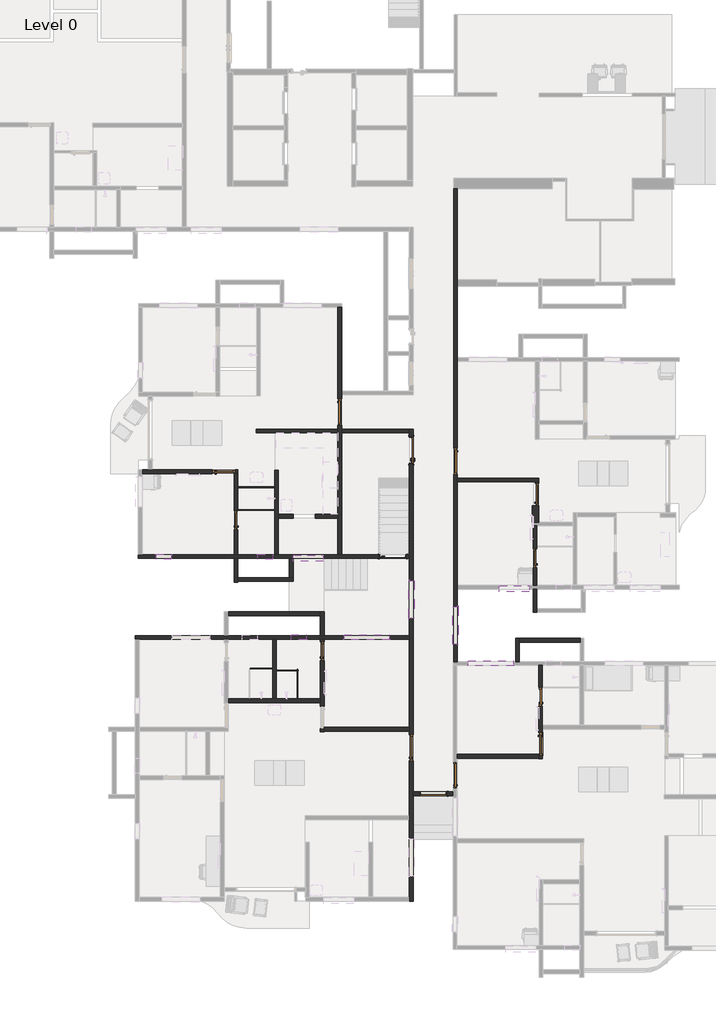
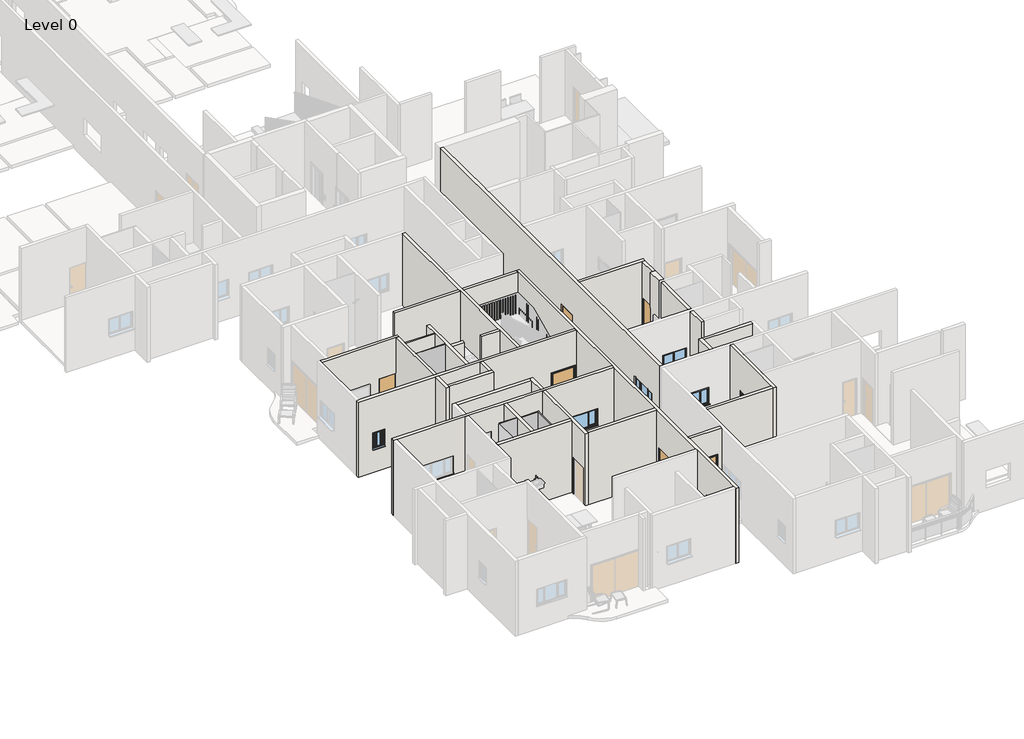
# One storey, part 2 of 14: 28 walls, 14 doors, 9 windows, 4 plates.
"""IFC4 building model written with IfcOpenShell, lengths in millimetres."""

from ifc_helpers import new_model, si_unit, frame, origin, origin_with_axes, place, context, project, spatial, polyline, outline, extrude, faceted_brep, transform, mapped, element, save
from components import doors_extsgl_flush_d1_30a970b5, doors_extsgl_flush_d1_11f69a25, doors_extsgl_flush_d2_fac1298c, doors_extsgl_flush_d2_5e0ff3e2, doors_extsgl_flush_d3_352cde1d, doors_extsgl_flush_d3_ba5ff989, doors_intsgl_3_75_1d728d0e, doors_intsgl_3_75_e7c258cb, system_panel_glazed_095a6893, system_panel_glazed_6806f88e, system_panel_glazed_1225bd09, system_panel_glazed_76c655e3, windows_concept_plain_dbl_4_d1e2e333, windows_sgl_plain_2_be143095, windows_tpl_variable_casement_2_47b04551, windows_tpl_variable_casement_5_ffad3fa3, windows_tpl_variable_casement_6_d811e495

model = new_model("IFC4")

# Units and contexts
model_context = context("Model", 3, world=origin())
ifc_project = project(units=[si_unit("LENGTHUNIT", "METRE", prefix="MILLI")], contexts=[model_context])

# Site, building, storey
site = spatial("IfcSite", under=ifc_project)
building = spatial("IfcBuilding", under=site)
storey = spatial("IfcBuildingStorey", under=building, Name="Level 0", Elevation=0.0)

# Doors
placement = place(None, origin())
doors_extsgl_flush_d1_shape = doors_extsgl_flush_d1_30a970b5(model_context)
element("IfcDoor", 1, ObjectType="Doors_ExtSgl_Flush : D1", at=placement, inside=storey, context=model_context, shape_type="MappedRepresentation", body=[
    mapped(doors_extsgl_flush_d1_shape, transform((-21668.1547508, 18097.2113431, 0.0), x_axis=(0.0, 1.0, 0.0), y_axis=(-1.0, 0.0, 0.0), z_axis=(0.0, 0.0, 1.0))),
])
element("IfcDoor", 2, ObjectType="Doors_ExtSgl_Flush : D1", at=placement, inside=storey, context=model_context, shape_type="MappedRepresentation", body=[
    mapped(doors_extsgl_flush_d1_shape, transform((-19869.6917798, 29735.6122683, 0.0), x_axis=(0.0, -1.0, 0.0), y_axis=(1.0, 0.0, 0.0), z_axis=(0.0, 0.0, 1.0))),
])
doors_extsgl_flush_d1_2_shape = doors_extsgl_flush_d1_11f69a25(model_context)
element("IfcDoor", 3, ObjectType="Doors_ExtSgl_Flush : D1", at=placement, inside=storey, context=model_context, shape_type="MappedRepresentation", body=[
    mapped(doors_extsgl_flush_d1_2_shape, transform((-19889.1949343, 16979.4762397, 0.0), x_axis=(0.0, 1.0, 0.0), y_axis=(-1.0, 0.0, 0.0), z_axis=(0.0, 0.0, 1.0))),
])
element("IfcDoor", 4, ObjectType="Doors_ExtSgl_Flush : D1", at=placement, inside=storey, context=model_context, shape_type="MappedRepresentation", body=[
    mapped(doors_extsgl_flush_d1_2_shape, transform((-24570.7800447, 31731.8982557, 0.0), x_axis=(0.0, -1.0, 0.0), y_axis=(1.0, 0.0, 0.0), z_axis=(0.0, 0.0, 1.0))),
])
doors_extsgl_flush_d2_shape = doors_extsgl_flush_d2_fac1298c(model_context)
element("IfcDoor", 5, ObjectType="Doors_ExtSgl_Flush : D2", at=placement, inside=storey, context=model_context, shape_type="MappedRepresentation", body=[
    mapped(doors_extsgl_flush_d2_shape, transform((-16561.3417798, 28376.6106683, 0.0), x_axis=(0.0, 1.0, 0.0), y_axis=(-1.0, 0.0, 0.0), z_axis=(0.0, 0.0, 1.0))),
])
doors_extsgl_flush_d2_2_shape = doors_extsgl_flush_d2_5e0ff3e2(model_context)
element("IfcDoor", 6, ObjectType="Doors_ExtSgl_Flush : D2", at=placement, inside=storey, context=model_context, shape_type="MappedRepresentation", body=[
    mapped(doors_extsgl_flush_d2_2_shape, transform((-16415.8741157, 18242.0106683, 0.0), x_axis=(0.0, -1.0, 0.0), y_axis=(1.0, 0.0, 0.0), z_axis=(0.0, 0.0, 1.0))),
])
element("IfcDoor", 7, ObjectType="Doors_ExtSgl_Flush : D2", at=placement, inside=storey, context=model_context, shape_type="MappedRepresentation", body=[
    mapped(doors_extsgl_flush_d2_2_shape, transform((-29288.9316447, 29306.9770746, 0.0), x_axis=(1.0, 0.0, 0.0), y_axis=(0.0, 1.0, 0.0), z_axis=(0.0, 0.0, 1.0))),
])
doors_extsgl_flush_d3_shape = doors_extsgl_flush_d3_352cde1d(model_context)
element("IfcDoor", 8, ObjectType="Doors_ExtSgl_Flush : D3", at=placement, inside=storey, context=model_context, shape_type="MappedRepresentation", body=[
    mapped(doors_extsgl_flush_d3_shape, transform((-25283.1553928, 22015.2629431, 0.0), x_axis=(0.0, 1.0, 0.0), y_axis=(-1.0, 0.0, 0.0), z_axis=(0.0, 0.0, 1.0))),
])
doors_extsgl_flush_d3_2_shape = doors_extsgl_flush_d3_ba5ff989(model_context)
element("IfcDoor", 9, ObjectType="Doors_ExtSgl_Flush : D3", at=placement, inside=storey, context=model_context, shape_type="MappedRepresentation", body=[
    mapped(doors_extsgl_flush_d3_2_shape, transform((-16415.8741157, 20166.1114683, 0.0), x_axis=(0.0, 1.0, 0.0), y_axis=(-1.0, 0.0, 0.0), z_axis=(0.0, 0.0, 1.0))),
])
element("IfcDoor", 10, ObjectType="Doors_ExtSgl_Flush : D3", at=placement, inside=storey, context=model_context, shape_type="MappedRepresentation", body=[
    mapped(doors_extsgl_flush_d3_2_shape, transform((-16639.8456172, 25796.359605, 0.0), x_axis=(0.0, 1.0, 0.0), y_axis=(-1.0, 0.0, 0.0), z_axis=(0.0, 0.0, 1.0))),
])
element("IfcDoor", 11, ObjectType="Doors_ExtSgl_Flush : D3", at=placement, inside=storey, context=model_context, shape_type="MappedRepresentation", body=[
    mapped(doors_extsgl_flush_d3_2_shape, transform((-28793.5300447, 27333.4986746, 0.0), x_axis=(0.0, 1.0, 0.0), y_axis=(-1.0, 0.0, 0.0), z_axis=(0.0, 0.0, 1.0))),
])
doors_intsgl_3_75_shape = doors_intsgl_3_75_1d728d0e(model_context)
element("IfcDoor", 12, ObjectType="Doors_IntSgl : 3.75'", at=placement, inside=storey, context=model_context, shape_type="MappedRepresentation", body=[
    mapped(doors_intsgl_3_75_shape, transform((-21668.1547508, 30185.5294818, 0.0), x_axis=(0.0, 1.0, 0.0), y_axis=(-1.0, 0.0, 0.0), z_axis=(0.0, 0.0, 1.0))),
])
element("IfcDoor", 13, ObjectType="Doors_IntSgl : 3.75'", at=placement, inside=storey, context=model_context, shape_type="MappedRepresentation", body=[
    mapped(doors_intsgl_3_75_shape, transform((-22417.4547508, 25858.9270746, 0.0), x_axis=(1.0, 0.0, 0.0), y_axis=(0.0, 1.0, 0.0), z_axis=(0.0, 0.0, 1.0))),
])
doors_intsgl_3_75_2_shape = doors_intsgl_3_75_e7c258cb(model_context)
element("IfcDoor", 14, ObjectType="Doors_IntSgl : 3.75'", at=placement, inside=storey, context=model_context, shape_type="MappedRepresentation", body=[
    mapped(doors_intsgl_3_75_2_shape, transform((-20778.6748425, 16225.043411, 508.0), x_axis=(-1.0, 0.0, 0.0), y_axis=(0.0, -1.0, 0.0), z_axis=(0.0, 0.0, 1.0))),
])

# Plates
system_panel_glazed_shape = system_panel_glazed_095a6893(model_context)
element("IfcPlate", 15, ObjectType="System Panel : Glazed", at=placement, inside=storey, context=model_context, shape_type="MappedRepresentation", body=[
    mapped(system_panel_glazed_shape, transform((-26257.0814081, 20677.4411882, 0.0), x_axis=(0.0, 1.0, 0.0), y_axis=(-1.0, 0.0, 0.0), z_axis=(0.0, 0.0, 1.0))),
])
system_panel_glazed_2_shape = system_panel_glazed_6806f88e(model_context)
element("IfcPlate", 16, ObjectType="System Panel : Glazed", at=placement, inside=storey, context=model_context, shape_type="MappedRepresentation", body=[
    mapped(system_panel_glazed_2_shape, transform((-27968.3995818, 27795.9116713, 0.0), x_axis=(-1.0, 0.0, 0.0), y_axis=(0.0, -1.0, 0.0), z_axis=(0.0, 0.0, 1.0))),
])
system_panel_glazed_3_shape = system_panel_glazed_1225bd09(model_context)
element("IfcPlate", 17, ObjectType="System Panel : Glazed", at=placement, inside=storey, context=model_context, shape_type="MappedRepresentation", body=[
    mapped(system_panel_glazed_3_shape, transform((-27760.3375826, 21274.3411882, 0.0), x_axis=(1.0, 0.0, 0.0), y_axis=(0.0, 1.0, 0.0), z_axis=(0.0, 0.0, 1.0))),
])
system_panel_glazed_4_shape = system_panel_glazed_76c655e3(model_context)
element("IfcPlate", 18, ObjectType="System Panel : Glazed", at=placement, inside=storey, context=model_context, shape_type="MappedRepresentation", body=[
    mapped(system_panel_glazed_4_shape, transform((-26705.9444157, 21274.3411882, 0.0), x_axis=(-1.0, 0.0, 0.0), y_axis=(0.0, -1.0, 0.0), z_axis=(0.0, 0.0, 1.0))),
])

# Walls
element("IfcWall", 19, ObjectType="W1", at=placement, inside=storey, context=model_context, shape_type="Brep", body=[
    faceted_brep([(-16492.0741157, 21442.5122683, 0.0), (-16492.0741157, 20547.1114683, 0.0), (-16492.0741157, 20547.1114683, 2110.0), (-16492.0741157, 19785.1114683, 2110.0), (-16492.0741157, 19785.1114683, 0.0), (-16492.0741157, 18699.2106683, 0.0), (-16492.0741157, 18699.2106683, 2110.0), (-16492.0741157, 17784.8106683, 2110.0), (-16492.0741157, 17784.8106683, 0.0), (-16492.0741157, 17670.5106683, 0.0), (-16492.0741157, 17651.5114683, 0.0), (-16492.0741157, 17651.5114683, 4000.0), (-16492.0741157, 17670.5106683, 4000.0), (-16492.0741157, 17822.9106683, 4000.0), (-16492.0741157, 21442.5122683, 4000.0), (-16339.6741157, 20547.1114683, 2110.0), (-16339.6741157, 20547.1114683, 0.0), (-16339.6741157, 21442.5122683, 0.0), (-16339.6741157, 21442.5122683, 4000.0), (-16339.6741157, 18997.7114683, 4000.0), (-16339.6741157, 18845.3114683, 4000.0), (-16339.6741157, 17651.5114683, 4000.0), (-16339.6741157, 17651.5114683, 0.0), (-16339.6741157, 17784.8106683, 0.0), (-16339.6741157, 17784.8106683, 2110.0), (-16339.6741157, 18699.2106683, 2110.0), (-16339.6741157, 18699.2106683, 0.0), (-16339.6741157, 18845.3114683, 0.0), (-16339.6741157, 18997.7114683, 0.0), (-16339.6741157, 19785.1114683, 0.0), (-16339.6741157, 19785.1114683, 2110.0)], [[[0, 1, 2, 3, 4, 5, 6, 7, 8, 9, 10, 11, 12, 13, 14]], [[15, 16, 17, 18, 19, 20, 21, 22, 23, 24, 25, 26, 27, 28, 29, 30]], [[10, 9, 8, 23, 22]], [[17, 16, 1, 0]], [[29, 28, 27, 26, 5, 4]], [[11, 10, 22, 21]], [[14, 13, 12, 11, 21, 20, 19, 18]], [[0, 14, 18, 17]], [[26, 25, 6, 5]], [[24, 23, 8, 7]], [[25, 24, 7, 6]], [[4, 3, 30, 29]], [[2, 1, 16, 15]], [[3, 2, 15, 30]]]),
])
element("IfcWall", 20, ObjectType="W1", at=placement, inside=storey, context=model_context, shape_type="Brep", body=[
    faceted_brep([(-19812.9949343, 17670.5106683, 0.0), (-16492.0741157, 17670.5106683, 0.0), (-16492.0741157, 17670.5106683, 4000.0), (-19812.9949343, 17670.5106683, 4000.0), (-19812.9949343, 17822.9106683, 0.0), (-19812.9949343, 17822.9106683, 4000.0), (-16492.0741157, 17822.9106683, 4000.0), (-16492.0741157, 17822.9106683, 0.0), (-16492.0741157, 17784.8106683, 0.0)], [[[0, 1, 2, 3]], [[4, 5, 6, 7]], [[1, 0, 4, 7, 8]], [[3, 2, 6, 5]], [[0, 3, 5, 4]], [[2, 1, 8, 7, 6]]]),
])
element("IfcWall", 21, ObjectType="W1", at=placement, inside=storey, context=model_context, shape_type="SweptSolid", body=[
    extrude(outline(polyline([(0.0, -21591.9547508), (0.0, -19965.3949343), (4000.0, -19965.3949343), (4000.0, -21591.9547508), (0.0, -21591.9547508)]), holes=[polyline([(508.0, -21350.1748425), (2641.6, -21350.1748425), (2641.6, -20207.1748425), (508.0, -20207.1748425), (508.0, -21350.1748425)])]), frame((0.0, 16148.843411, 0.0), z_axis=(0.0, 1.0, 0.0), x_axis=(0.0, 0.0, 1.0)), (0.0, 0.0, 1.0), 152.4),
])
element("IfcWall", 22, ObjectType="W1", at=placement, inside=storey, context=model_context, shape_type="Brep", body=[
    faceted_brep([(-21591.9547508, 31036.4294818, 4000.0), (-21591.9547508, 16301.243411, 4000.0), (-21591.9547508, 16148.843411, 4000.0), (-21591.9547508, 11859.4294818, 4000.0), (-21591.9547508, 11859.4294818, 0.0), (-21591.9547508, 16148.843411, 0.0), (-21591.9547508, 16301.243411, 0.0), (-21591.9547508, 17563.8113431, 0.0), (-21591.9547508, 17563.8113431, 2110.0), (-21591.9547508, 18630.6113431, 2110.0), (-21591.9547508, 18630.6113431, 0.0), (-21591.9547508, 29614.0294818, 0.0), (-21591.9547508, 29614.0294818, 2133.6), (-21591.9547508, 30757.0294818, 2133.6), (-21591.9547508, 30757.0294818, 0.0), (-21591.9547508, 31036.4294818, 0.0), (-21591.9547508, 14397.2288681, 2110.0), (-21591.9547508, 14397.2288681, 1200.0), (-21591.9547508, 12873.2288681, 1200.0), (-21591.9547508, 12873.2288681, 2110.0), (-21591.9547508, 24887.7601529, 2110.0), (-21591.9547508, 24887.7601529, 1200.0), (-21591.9547508, 23363.7601529, 1200.0), (-21591.9547508, 23363.7601529, 2110.0), (-21744.3547508, 11859.4294818, 4000.0), (-21744.3547508, 12011.8294818, 4000.0), (-21744.3547508, 15172.0304681, 4000.0), (-21744.3547508, 15324.4304681, 4000.0), (-21744.3547508, 18770.4129431, 4000.0), (-21744.3547508, 18922.8129431, 4000.0), (-21744.3547508, 22500.1601529, 4000.0), (-21744.3547508, 22652.5601529, 4000.0), (-21744.3547508, 25782.7270746, 4000.0), (-21744.3547508, 25935.1270746, 4000.0), (-21744.3547508, 30884.0294818, 4000.0), (-21744.3547508, 31036.4294818, 4000.0), (-21744.3547508, 31036.4294818, 0.0), (-21744.3547508, 30884.0294818, 0.0), (-21744.3547508, 30757.0294818, 0.0), (-21744.3547508, 30757.0294818, 2133.6), (-21744.3547508, 29614.0294818, 2133.6), (-21744.3547508, 29614.0294818, 0.0), (-21744.3547508, 25935.1270746, 0.0), (-21744.3547508, 25782.7270746, 0.0), (-21744.3547508, 22652.5601529, 0.0), (-21744.3547508, 22500.1601529, 0.0), (-21744.3547508, 18922.8129431, 0.0), (-21744.3547508, 18770.4129431, 0.0), (-21744.3547508, 18630.6113431, 0.0), (-21744.3547508, 18630.6113431, 2110.0), (-21744.3547508, 17563.8113431, 2110.0), (-21744.3547508, 17563.8113431, 0.0), (-21744.3547508, 15324.4304681, 0.0), (-21744.3547508, 15172.0304681, 0.0), (-21744.3547508, 12011.8294818, 0.0), (-21744.3547508, 11859.4294818, 0.0), (-21744.3547508, 14397.2288681, 2110.0), (-21744.3547508, 12873.2288681, 2110.0), (-21744.3547508, 12873.2288681, 1200.0), (-21744.3547508, 14397.2288681, 1200.0), (-21744.3547508, 24887.7601529, 2110.0), (-21744.3547508, 23363.7601529, 2110.0), (-21744.3547508, 23363.7601529, 1200.0), (-21744.3547508, 24887.7601529, 1200.0)], [[[0, 1, 2, 3, 4, 5, 6, 7, 8, 9, 10, 11, 12, 13, 14, 15], [16, 17, 18, 19], [20, 21, 22, 23]], [[24, 25, 26, 27, 28, 29, 30, 31, 32, 33, 34, 35, 36, 37, 38, 39, 40, 41, 42, 43, 44, 45, 46, 47, 48, 49, 50, 51, 52, 53, 54, 55], [56, 57, 58, 59], [60, 61, 62, 63]], [[4, 55, 54, 53, 52, 51, 7, 6, 5]], [[36, 15, 14, 38, 37]], [[10, 48, 47, 46, 45, 44, 43, 42, 41, 11]], [[3, 2, 1, 0, 35, 34, 33, 32, 31, 30, 29, 28, 27, 26, 25, 24]], [[4, 3, 24, 55]], [[0, 15, 36, 35]], [[51, 50, 8, 7]], [[49, 48, 10, 9]], [[50, 49, 9, 8]], [[17, 16, 56, 59]], [[18, 17, 59, 58]], [[19, 18, 58, 57]], [[16, 19, 57, 56]], [[13, 39, 38, 14]], [[39, 13, 12, 40]], [[40, 12, 11, 41]], [[21, 20, 60, 63]], [[22, 21, 63, 62]], [[23, 22, 62, 61]], [[20, 23, 61, 60]]]),
])
element("IfcWall", 23, ObjectType="W1", at=placement, inside=storey, context=model_context, shape_type="Brep", body=[
    faceted_brep([(-21744.3547508, 22652.5601529, 0.0), (-25206.9553928, 22652.5601529, 0.0), (-25359.3553928, 22652.5601529, 0.0), (-29107.0280604, 22652.5601529, 0.0), (-29259.4280604, 22652.5601529, 0.0), (-32875.9555508, 22652.5601529, 0.0), (-32875.9555508, 22652.5601529, 4000.0), (-29259.4280604, 22652.5601529, 4000.0), (-29107.0280604, 22652.5601529, 4000.0), (-25359.3553928, 22652.5601529, 4000.0), (-25206.9553928, 22652.5601529, 4000.0), (-21744.3547508, 22652.5601529, 4000.0), (-28539.2090234, 22652.5601529, 2738.9328), (-28539.2090234, 22652.5601529, 1828.9328), (-27929.6090234, 22652.5601529, 1828.9328), (-27929.6090234, 22652.5601529, 2738.9328), (-26545.2074234, 22652.5601529, 2738.9328), (-26545.2074234, 22652.5601529, 1828.9328), (-25935.6074234, 22652.5601529, 1828.9328), (-25935.6074234, 22652.5601529, 2738.9328), (-31387.0322871, 22652.5601529, 2110.0), (-31387.0322871, 22652.5601529, 1200.0), (-29863.0322871, 22652.5601529, 1200.0), (-29863.0322871, 22652.5601529, 2110.0), (-24398.7563508, 22652.5601529, 2110.0), (-24398.7563508, 22652.5601529, 1200.0), (-22569.9563508, 22652.5601529, 1200.0), (-22569.9563508, 22652.5601529, 2110.0), (-21744.3547508, 22500.1601529, 0.0), (-21744.3547508, 22500.1601529, 4000.0), (-25206.9553928, 22500.1601529, 4000.0), (-25359.3553928, 22500.1601529, 4000.0), (-27154.8074234, 22500.1601529, 4000.0), (-27307.2074234, 22500.1601529, 4000.0), (-29107.0280604, 22500.1601529, 4000.0), (-29259.4280604, 22500.1601529, 4000.0), (-32723.5555508, 22500.1601529, 4000.0), (-32875.9555508, 22500.1601529, 4000.0), (-32875.9555508, 22500.1601529, 0.0), (-32723.5555508, 22500.1601529, 0.0), (-29259.4280604, 22500.1601529, 0.0), (-29107.0280604, 22500.1601529, 0.0), (-27307.2074234, 22500.1601529, 0.0), (-27154.8074234, 22500.1601529, 0.0), (-25359.3553928, 22500.1601529, 0.0), (-25206.9553928, 22500.1601529, 0.0), (-28539.2090234, 22500.1601529, 2738.9328), (-27929.6090234, 22500.1601529, 2738.9328), (-27929.6090234, 22500.1601529, 1828.9328), (-28539.2090234, 22500.1601529, 1828.9328), (-26545.2074234, 22500.1601529, 2738.9328), (-25935.6074234, 22500.1601529, 2738.9328), (-25935.6074234, 22500.1601529, 1828.9328), (-26545.2074234, 22500.1601529, 1828.9328), (-31387.0322871, 22500.1601529, 2110.0), (-29863.0322871, 22500.1601529, 2110.0), (-29863.0322871, 22500.1601529, 1200.0), (-31387.0322871, 22500.1601529, 1200.0), (-24398.7563508, 22500.1601529, 2110.0), (-22569.9563508, 22500.1601529, 2110.0), (-22569.9563508, 22500.1601529, 1200.0), (-24398.7563508, 22500.1601529, 1200.0)], [[[0, 1, 2, 3, 4, 5, 6, 7, 8, 9, 10, 11], [12, 13, 14, 15], [16, 17, 18, 19], [20, 21, 22, 23], [24, 25, 26, 27]], [[28, 29, 30, 31, 32, 33, 34, 35, 36, 37, 38, 39, 40, 41, 42, 43, 44, 45], [46, 47, 48, 49], [50, 51, 52, 53], [54, 55, 56, 57], [58, 59, 60, 61]], [[5, 4, 3, 2, 1, 0, 28, 45, 44, 43, 42, 41, 40, 39, 38]], [[11, 10, 9, 8, 7, 6, 37, 36, 35, 34, 33, 32, 31, 30, 29]], [[0, 11, 29, 28]], [[6, 5, 38, 37]], [[13, 12, 46, 49]], [[14, 13, 49, 48]], [[15, 14, 48, 47]], [[12, 15, 47, 46]], [[17, 16, 50, 53]], [[18, 17, 53, 52]], [[19, 18, 52, 51]], [[16, 19, 51, 50]], [[21, 20, 54, 57]], [[22, 21, 57, 56]], [[23, 22, 56, 55]], [[20, 23, 55, 54]], [[25, 24, 58, 61]], [[26, 25, 61, 60]], [[27, 26, 60, 59]], [[24, 27, 59, 58]]]),
])
element("IfcWall", 24, ObjectType="W1", at=placement, inside=storey, context=model_context, shape_type="Brep", body=[
    faceted_brep([(-29107.0280604, 19928.1411882, 0.0), (-25359.3553928, 19928.1411882, 0.0), (-25359.3553928, 19928.1411882, 4000.0), (-29107.0280604, 19928.1411882, 4000.0), (-29107.0280604, 20080.5411882, 0.0), (-29107.0280604, 20080.5411882, 4000.0), (-27307.2074234, 20080.5411882, 4000.0), (-27154.8074234, 20080.5411882, 4000.0), (-25359.3553928, 20080.5411882, 4000.0), (-25359.3553928, 20080.5411882, 0.0), (-27154.8074234, 20080.5411882, 0.0), (-27307.2074234, 20080.5411882, 0.0)], [[[0, 1, 2, 3]], [[4, 5, 6, 7, 8, 9, 10, 11]], [[1, 0, 4, 11, 10, 9]], [[3, 2, 8, 7, 6, 5]], [[0, 3, 5, 4]], [[2, 1, 9, 8]]]),
])
element("IfcWall", 25, ObjectType="W1", at=placement, inside=storey, context=model_context, shape_type="SweptSolid", body=[
    extrude(outline(polyline([(-27307.2074234, 20080.5411882), (-27307.2074234, 22500.1601529), (-27154.8074234, 22500.1601529), (-27154.8074234, 20080.5411882), (-27307.2074234, 20080.5411882)])), origin_with_axes(), (0.0, 0.0, 1.0), 4000.0),
])
element("IfcWall", 26, ObjectType="W1", at=placement, inside=storey, context=model_context, shape_type="Brep", body=[
    faceted_brep([(-25359.3553928, 18745.0129431, 0.0), (-25359.3553928, 18745.0129431, 4000.0), (-25359.3553928, 19928.1411882, 4000.0), (-25359.3553928, 20080.5411882, 4000.0), (-25359.3553928, 22500.1601529, 4000.0), (-25359.3553928, 22500.1601529, 0.0), (-25359.3553928, 22396.2629431, 0.0), (-25359.3553928, 22396.2629431, 2110.0), (-25359.3553928, 21634.2629431, 2110.0), (-25359.3553928, 21634.2629431, 0.0), (-25359.3553928, 20080.5411882, 0.0), (-25359.3553928, 19928.1411882, 0.0), (-25359.3553928, 19787.3762656, 0.0), (-25359.3553928, 19787.3762656, 2110.0), (-25359.3553928, 18872.9762656, 2110.0), (-25359.3553928, 18872.9762656, 0.0), (-25206.9553928, 18745.0129431, 4000.0), (-25206.9553928, 18745.0129431, 0.0), (-25206.9553928, 18770.4129431, 0.0), (-25206.9553928, 18872.9762656, 0.0), (-25206.9553928, 18872.9762656, 2110.0), (-25206.9553928, 19787.3762656, 2110.0), (-25206.9553928, 19787.3762656, 0.0), (-25206.9553928, 21634.2629431, 0.0), (-25206.9553928, 21634.2629431, 2110.0), (-25206.9553928, 22396.2629431, 2110.0), (-25206.9553928, 22396.2629431, 0.0), (-25206.9553928, 22500.1601529, 0.0), (-25206.9553928, 22500.1601529, 4000.0), (-25206.9553928, 18922.8129431, 4000.0), (-25206.9553928, 18770.4129431, 4000.0)], [[[0, 1, 2, 3, 4, 5, 6, 7, 8, 9, 10, 11, 12, 13, 14, 15]], [[16, 17, 18, 19, 20, 21, 22, 23, 24, 25, 26, 27, 28, 29, 30]], [[17, 0, 15, 19, 18]], [[22, 12, 11, 10, 9, 23]], [[26, 6, 5, 27]], [[1, 0, 17, 16]], [[1, 16, 30, 29, 28, 4, 3, 2]], [[5, 4, 28, 27]], [[22, 21, 13, 12]], [[20, 19, 15, 14]], [[21, 20, 14, 13]], [[9, 8, 24, 23]], [[7, 6, 26, 25]], [[8, 7, 25, 24]]]),
    faceted_brep([(-25359.3553928, 23611.1411882, 4000.0), (-25359.3553928, 23611.1411882, 0.0), (-25359.3553928, 23458.7411882, 0.0), (-25359.3553928, 22652.5601529, 0.0), (-25359.3553928, 22652.5601529, 4000.0), (-25359.3553928, 23458.7411882, 4000.0), (-25206.9553928, 23611.1411882, 0.0), (-25206.9553928, 23611.1411882, 4000.0), (-25206.9553928, 22652.5601529, 4000.0), (-25206.9553928, 22652.5601529, 0.0)], [[[0, 1, 2, 3, 4, 5]], [[6, 7, 8, 9]], [[1, 6, 9, 3, 2]], [[7, 0, 5, 4, 8]], [[4, 3, 9, 8]], [[1, 0, 7, 6]]]),
])
element("IfcWall", 27, ObjectType="W1", at=placement, inside=storey, context=model_context, shape_type="Brep", body=[
    faceted_brep([(-25206.9553928, 18770.4129431, 0.0), (-21744.3547508, 18770.4129431, 0.0), (-21744.3547508, 18770.4129431, 4000.0), (-25206.9553928, 18770.4129431, 4000.0), (-25206.9553928, 18922.8129431, 0.0), (-25206.9553928, 18922.8129431, 4000.0), (-21744.3547508, 18922.8129431, 4000.0), (-21744.3547508, 18922.8129431, 0.0), (-25206.9553928, 18872.9762656, 0.0)], [[[0, 1, 2, 3]], [[4, 5, 6, 7]], [[1, 0, 8, 4, 7]], [[3, 2, 6, 5]], [[2, 1, 7, 6]], [[0, 3, 5, 4, 8]]]),
])
element("IfcWall", 28, ObjectType="W1", at=placement, inside=storey, context=model_context, shape_type="Brep", body=[
    faceted_brep([(-32762.2800447, 25935.1270746, 4000.0), (-32609.8800447, 25935.1270746, 4000.0), (-28869.7300447, 25935.1270746, 4000.0), (-28717.3300447, 25935.1270746, 4000.0), (-27219.4691188, 25935.1270746, 4000.0), (-27067.0691188, 25935.1270746, 4000.0), (-24646.9800447, 25935.1270746, 4000.0), (-24494.5800447, 25935.1270746, 4000.0), (-21744.3547508, 25935.1270746, 4000.0), (-21744.3547508, 25935.1270746, 0.0), (-21845.9547508, 25935.1270746, 0.0), (-21845.9547508, 25935.1270746, 2133.6), (-22988.9547508, 25935.1270746, 2133.6), (-22988.9547508, 25935.1270746, 0.0), (-24494.5800447, 25935.1270746, 0.0), (-24646.9800447, 25935.1270746, 0.0), (-27067.0691188, 25935.1270746, 0.0), (-27219.4691188, 25935.1270746, 0.0), (-28717.3300447, 25935.1270746, 0.0), (-28869.7300447, 25935.1270746, 0.0), (-32609.8800447, 25935.1270746, 0.0), (-32762.2800447, 25935.1270746, 0.0), (-31416.0800447, 25935.1270746, 2110.0), (-32025.6800447, 25935.1270746, 2110.0), (-32025.6800447, 25935.1270746, 1200.0), (-31416.0800447, 25935.1270746, 1200.0), (-25247.4245818, 25935.1270746, 2110.0), (-26466.6245818, 25935.1270746, 2110.0), (-26466.6245818, 25935.1270746, 1200.0), (-25247.4245818, 25935.1270746, 1200.0), (-27295.6691188, 25935.1270746, 1828.9328), (-27295.6691188, 25935.1270746, 2738.9328), (-27905.2691188, 25935.1270746, 2738.9328), (-27905.2691188, 25935.1270746, 1828.9328), (-21744.3547508, 25782.7270746, 4000.0), (-26469.4300447, 25782.7270746, 4000.0), (-26621.8300447, 25782.7270746, 4000.0), (-28717.3300447, 25782.7270746, 4000.0), (-28869.7300447, 25782.7270746, 4000.0), (-32762.2800447, 25782.7270746, 4000.0), (-32762.2800447, 25782.7270746, 0.0), (-28869.7300447, 25782.7270746, 0.0), (-28717.3300447, 25782.7270746, 0.0), (-26621.8300447, 25782.7270746, 0.0), (-26469.4300447, 25782.7270746, 0.0), (-22988.9547508, 25782.7270746, 0.0), (-22988.9547508, 25782.7270746, 2133.6), (-21845.9547508, 25782.7270746, 2133.6), (-21845.9547508, 25782.7270746, 0.0), (-21744.3547508, 25782.7270746, 0.0), (-31416.0800447, 25782.7270746, 2110.0), (-31416.0800447, 25782.7270746, 1200.0), (-32025.6800447, 25782.7270746, 1200.0), (-32025.6800447, 25782.7270746, 2110.0), (-25247.4245818, 25782.7270746, 2110.0), (-25247.4245818, 25782.7270746, 1200.0), (-26466.6245818, 25782.7270746, 1200.0), (-26466.6245818, 25782.7270746, 2110.0), (-27295.6691188, 25782.7270746, 2738.9328), (-27295.6691188, 25782.7270746, 1828.9328), (-27905.2691188, 25782.7270746, 1828.9328), (-27905.2691188, 25782.7270746, 2738.9328)], [[[0, 1, 2, 3, 4, 5, 6, 7, 8, 9, 10, 11, 12, 13, 14, 15, 16, 17, 18, 19, 20, 21], [22, 23, 24, 25], [26, 27, 28, 29], [30, 31, 32, 33]], [[34, 35, 36, 37, 38, 39, 40, 41, 42, 43, 44, 45, 46, 47, 48, 49], [50, 51, 52, 53], [54, 55, 56, 57], [58, 59, 60, 61]], [[40, 21, 20, 19, 18, 17, 16, 15, 14, 13, 45, 44, 43, 42, 41]], [[9, 49, 48, 10]], [[8, 7, 6, 5, 4, 3, 2, 1, 0, 39, 38, 37, 36, 35, 34]], [[0, 21, 40, 39]], [[51, 50, 22, 25]], [[52, 51, 25, 24]], [[53, 52, 24, 23]], [[50, 53, 23, 22]], [[55, 54, 26, 29]], [[56, 55, 29, 28]], [[57, 56, 28, 27]], [[54, 57, 27, 26]], [[59, 58, 31, 30]], [[60, 59, 30, 33]], [[61, 60, 33, 32]], [[58, 61, 32, 31]], [[9, 8, 34, 49]], [[47, 11, 10, 48]], [[11, 47, 46, 12]], [[12, 46, 45, 13]]]),
])
element("IfcWall", 29, ObjectType="W1", at=placement, inside=storey, context=model_context, shape_type="Brep", body=[
    faceted_brep([(-24494.5800447, 25935.1270746, 0.0), (-24494.5800447, 30884.0294818, 0.0), (-24494.5800447, 31036.4294818, 0.0), (-24494.5800447, 31198.4982557, 0.0), (-24494.5800447, 31198.4982557, 2110.0), (-24494.5800447, 32265.2982557, 2110.0), (-24494.5800447, 32265.2982557, 0.0), (-24494.5800447, 32430.4998557, 0.0), (-24494.5800447, 32582.8998557, 0.0), (-24494.5800447, 35984.9800488, 0.0), (-24494.5800447, 35984.9800488, 4000.0), (-24494.5800447, 32582.8998557, 4000.0), (-24494.5800447, 32430.4998557, 4000.0), (-24494.5800447, 31036.4294818, 4000.0), (-24494.5800447, 30884.0294818, 4000.0), (-24494.5800447, 25935.1270746, 4000.0), (-24646.9800447, 31198.4982557, 2110.0), (-24646.9800447, 31198.4982557, 0.0), (-24646.9800447, 31036.4294818, 0.0), (-24646.9800447, 30884.0294818, 0.0), (-24646.9800447, 27580.0116713, 0.0), (-24646.9800447, 27427.6116713, 0.0), (-24646.9800447, 25935.1270746, 0.0), (-24646.9800447, 25935.1270746, 4000.0), (-24646.9800447, 27427.6116713, 4000.0), (-24646.9800447, 27580.0116713, 4000.0), (-24646.9800447, 30884.0294818, 4000.0), (-24646.9800447, 31036.4294818, 4000.0), (-24646.9800447, 35984.9800488, 4000.0), (-24646.9800447, 35984.9800488, 0.0), (-24646.9800447, 32265.2982557, 0.0), (-24646.9800447, 32265.2982557, 2110.0)], [[[0, 1, 2, 3, 4, 5, 6, 7, 8, 9, 10, 11, 12, 13, 14, 15]], [[16, 17, 18, 19, 20, 21, 22, 23, 24, 25, 26, 27, 28, 29, 30, 31]], [[30, 29, 9, 8, 7, 6]], [[22, 21, 20, 19, 18, 17, 3, 2, 1, 0]], [[15, 14, 13, 12, 11, 10, 28, 27, 26, 25, 24, 23]], [[0, 15, 23, 22]], [[10, 9, 29, 28]], [[6, 5, 31, 30]], [[4, 3, 17, 16]], [[5, 4, 16, 31]]]),
])
element("IfcWall", 30, ObjectType="W1", at=placement, inside=storey, context=model_context, shape_type="SweptSolid", body=[
    extrude(outline(polyline([(-27961.1063508, 30884.0294818), (-27961.1063508, 31036.4294818), (-24646.9800447, 31036.4294818), (-24646.9800447, 30884.0294818), (-27961.1063508, 30884.0294818)])), origin_with_axes(), (0.0, 0.0, 1.0), 4000.0),
    extrude(outline(polyline([(-21744.3547508, 31036.4294818), (-21744.3547508, 30884.0294818), (-24494.5800447, 30884.0294818), (-24494.5800447, 31036.4294818), (-21744.3547508, 31036.4294818)])), origin_with_axes(), (0.0, 0.0, 1.0), 4000.0),
])
element("IfcWall", 31, ObjectType="W1", at=placement, inside=storey, context=model_context, shape_type="Brep", body=[
    faceted_brep([(-28831.7316447, 29230.7770746, 2110.0), (-28831.7316447, 29230.7770746, 0.0), (-28717.3300447, 29230.7770746, 0.0), (-28717.3300447, 29230.7770746, 4000.0), (-28869.7300447, 29230.7770746, 4000.0), (-32609.8800447, 29230.7770746, 4000.0), (-32609.8800447, 29230.7770746, 0.0), (-29746.1316447, 29230.7770746, 0.0), (-29746.1316447, 29230.7770746, 2110.0), (-28717.3300447, 29383.1770746, 0.0), (-28831.7316447, 29383.1770746, 0.0), (-28831.7316447, 29383.1770746, 2110.0), (-29746.1316447, 29383.1770746, 2110.0), (-29746.1316447, 29383.1770746, 0.0), (-32203.4800447, 29383.1770746, 0.0), (-32355.8800447, 29383.1770746, 0.0), (-32609.8800447, 29383.1770746, 0.0), (-32609.8800447, 29383.1770746, 4000.0), (-32355.8800447, 29383.1770746, 4000.0), (-32203.4800447, 29383.1770746, 4000.0), (-28717.3300447, 29383.1770746, 4000.0)], [[[0, 1, 2, 3, 4, 5, 6, 7, 8]], [[9, 10, 11, 12, 13, 14, 15, 16, 17, 18, 19, 20]], [[7, 6, 16, 15, 14, 13]], [[2, 1, 10, 9]], [[5, 4, 3, 20, 19, 18, 17]], [[6, 5, 17, 16]], [[3, 2, 9, 20]], [[13, 12, 8, 7]], [[11, 10, 1, 0]], [[12, 11, 0, 8]]]),
])
element("IfcWall", 32, ObjectType="W1", at=placement, inside=storey, context=model_context, shape_type="Brep", body=[
    faceted_brep([(-28869.7300447, 24823.8262746, 0.0), (-28869.7300447, 24823.8262746, 4000.0), (-28869.7300447, 25782.7270746, 4000.0), (-28869.7300447, 25782.7270746, 0.0), (-28717.3300447, 24823.8262746, 4000.0), (-28717.3300447, 24823.8262746, 0.0), (-28717.3300447, 24849.2262746, 0.0), (-28717.3300447, 25001.6262746, 0.0), (-28717.3300447, 25782.7270746, 0.0), (-28717.3300447, 25782.7270746, 4000.0), (-28717.3300447, 25001.6262746, 4000.0), (-28717.3300447, 24849.2262746, 4000.0)], [[[0, 1, 2, 3]], [[4, 5, 6, 7, 8, 9, 10, 11]], [[5, 0, 3, 8, 7, 6]], [[1, 0, 5, 4]], [[1, 4, 11, 10, 9, 2]], [[3, 2, 9, 8]]]),
    faceted_brep([(-28869.7300447, 29230.7770746, 4000.0), (-28869.7300447, 29230.7770746, 0.0), (-28869.7300447, 27714.4986746, 0.0), (-28869.7300447, 27714.4986746, 2110.0), (-28869.7300447, 26952.4986746, 2110.0), (-28869.7300447, 26952.4986746, 0.0), (-28869.7300447, 25935.1270746, 0.0), (-28869.7300447, 25935.1270746, 4000.0), (-28717.3300447, 29230.7770746, 0.0), (-28717.3300447, 29230.7770746, 4000.0), (-28717.3300447, 28703.6762746, 4000.0), (-28717.3300447, 28654.2986746, 4000.0), (-28717.3300447, 25935.1270746, 4000.0), (-28717.3300447, 25935.1270746, 0.0), (-28717.3300447, 26952.4986746, 0.0), (-28717.3300447, 26952.4986746, 2110.0), (-28717.3300447, 27714.4986746, 2110.0), (-28717.3300447, 27714.4986746, 0.0), (-28717.3300447, 28654.2986746, 0.0), (-28717.3300447, 28703.6762746, 0.0), (-28831.7316447, 29230.7770746, 0.0)], [[[0, 1, 2, 3, 4, 5, 6, 7]], [[8, 9, 10, 11, 12, 13, 14, 15, 16, 17, 18, 19]], [[1, 20, 8, 19, 18, 17, 2]], [[5, 14, 13, 6]], [[9, 0, 7, 12, 11, 10]], [[1, 0, 9, 8, 20]], [[7, 6, 13, 12]], [[5, 4, 15, 14]], [[3, 2, 17, 16]], [[4, 3, 16, 15]]]),
])
element("IfcWall", 33, ObjectType="W1", at=placement, inside=storey, context=model_context, shape_type="Brep", body=[
    faceted_brep([(-28717.3300447, 24849.2262746, 0.0), (-26469.4300447, 24849.2262746, 0.0), (-26469.4300447, 24849.2262746, 4000.0), (-28717.3300447, 24849.2262746, 4000.0), (-28717.3300447, 25001.6262746, 0.0), (-28717.3300447, 25001.6262746, 4000.0), (-26621.8300447, 25001.6262746, 4000.0), (-26469.4300447, 25001.6262746, 4000.0), (-26469.4300447, 25001.6262746, 0.0), (-26621.8300447, 25001.6262746, 0.0)], [[[0, 1, 2, 3]], [[4, 5, 6, 7, 8, 9]], [[1, 0, 4, 9, 8]], [[3, 2, 7, 6, 5]], [[0, 3, 5, 4]], [[2, 1, 8, 7]]]),
])
element("IfcWall", 34, ObjectType="W1", at=placement, inside=storey, context=model_context, shape_type="SweptSolid", body=[
    extrude(outline(polyline([(-26469.4300447, 25782.7270746), (-26469.4300447, 25001.6262746), (-26621.8300447, 25001.6262746), (-26621.8300447, 25782.7270746), (-26469.4300447, 25782.7270746)])), origin_with_axes(), (0.0, 0.0, 1.0), 4000.0),
])
element("IfcWall", 35, ObjectType="W1", at=placement, inside=storey, context=model_context, shape_type="Brep", body=[
    faceted_brep([(-27219.4691188, 29369.8991476, 0.0), (-27219.4691188, 28703.6762746, 0.0), (-27219.4691188, 28654.2986746, 0.0), (-27219.4691188, 25935.1270746, 0.0), (-27219.4691188, 25935.1270746, 4000.0), (-27219.4691188, 28654.2986746, 4000.0), (-27219.4691188, 28703.6762746, 4000.0), (-27219.4691188, 29369.8991476, 4000.0), (-27067.0691188, 29369.8991476, 0.0), (-27067.0691188, 29369.8991476, 4000.0), (-27067.0691188, 27580.0116713, 4000.0), (-27067.0691188, 27427.6116713, 4000.0), (-27067.0691188, 25935.1270746, 4000.0), (-27067.0691188, 25935.1270746, 0.0), (-27067.0691188, 27427.6116713, 0.0), (-27067.0691188, 27580.0116713, 0.0)], [[[0, 1, 2, 3, 4, 5, 6, 7]], [[8, 9, 10, 11, 12, 13, 14, 15]], [[3, 2, 1, 0, 8, 15, 14, 13]], [[7, 6, 5, 4, 12, 11, 10, 9]], [[0, 7, 9, 8]], [[4, 3, 13, 12]]]),
])
element("IfcWall", 36, ObjectType="W1", at=placement, inside=storey, context=model_context, shape_type="Brep", body=[
    faceted_brep([(-19793.4917798, 21594.9122683, 0.0), (-19793.4917798, 24541.3122683, 0.0), (-19793.4917798, 24693.7122683, 0.0), (-19793.4917798, 28897.4122683, 0.0), (-19793.4917798, 29049.8122683, 0.0), (-19793.4917798, 29202.2122683, 0.0), (-19793.4917798, 29202.2122683, 2110.0), (-19793.4917798, 30269.0122683, 2110.0), (-19793.4917798, 30269.0122683, 0.0), (-19793.4917798, 33786.9122683, 0.0), (-19793.4917798, 33939.3122683, 0.0), (-19793.4917798, 36847.7267386, 0.0), (-19793.4917798, 37108.0259386, 0.0), (-19793.4917798, 40796.435929, 0.0), (-19793.4917798, 40796.435929, 4000.0), (-19793.4917798, 37108.0259386, 4000.0), (-19793.4917798, 36847.7267386, 4000.0), (-19793.4917798, 33939.3122683, 4000.0), (-19793.4917798, 33786.9122683, 4000.0), (-19793.4917798, 29049.8122683, 4000.0), (-19793.4917798, 28897.4122683, 4000.0), (-19793.4917798, 24693.7122683, 4000.0), (-19793.4917798, 24541.3122683, 4000.0), (-19793.4917798, 21594.9122683, 4000.0), (-19793.4917798, 22306.1122683, 2110.0), (-19793.4917798, 23830.1122683, 2110.0), (-19793.4917798, 23830.1122683, 1200.0), (-19793.4917798, 22306.1122683, 1200.0), (-19945.8917798, 29202.2122683, 2110.0), (-19945.8917798, 29202.2122683, 0.0), (-19945.8917798, 21594.9122683, 0.0), (-19945.8917798, 21594.9122683, 4000.0), (-19945.8917798, 40796.435929, 4000.0), (-19945.8917798, 40796.435929, 0.0), (-19945.8917798, 30269.0122683, 0.0), (-19945.8917798, 30269.0122683, 2110.0), (-19945.8917798, 22306.1122683, 2110.0), (-19945.8917798, 22306.1122683, 1200.0), (-19945.8917798, 23830.1122683, 1200.0), (-19945.8917798, 23830.1122683, 2110.0)], [[[0, 1, 2, 3, 4, 5, 6, 7, 8, 9, 10, 11, 12, 13, 14, 15, 16, 17, 18, 19, 20, 21, 22, 23], [24, 25, 26, 27]], [[28, 29, 30, 31, 32, 33, 34, 35], [36, 37, 38, 39]], [[34, 33, 13, 12, 11, 10, 9, 8]], [[30, 29, 5, 4, 3, 2, 1, 0]], [[23, 22, 21, 20, 19, 18, 17, 16, 15, 14, 32, 31]], [[0, 23, 31, 30]], [[14, 13, 33, 32]], [[8, 7, 35, 34]], [[6, 5, 29, 28]], [[7, 6, 28, 35]], [[37, 36, 24, 27]], [[38, 37, 27, 26]], [[39, 38, 26, 25]], [[36, 39, 25, 24]]]),
])
element("IfcWall", 37, ObjectType="W1", at=placement, inside=storey, context=model_context, shape_type="Brep", body=[
    faceted_brep([(-17277.7094141, 21594.9122683, 0.0), (-17277.7094141, 22382.3122683, 0.0), (-17277.7094141, 22534.7122683, 0.0), (-17277.7094141, 22534.7122683, 4000.0), (-17277.7094141, 22382.3122683, 4000.0), (-17277.7094141, 21594.9122683, 4000.0), (-17430.1094141, 21594.9122683, 0.0), (-17430.1094141, 21594.9122683, 4000.0), (-17430.1094141, 22534.7122683, 4000.0), (-17430.1094141, 22534.7122683, 0.0)], [[[0, 1, 2, 3, 4, 5]], [[6, 7, 8, 9]], [[2, 1, 0, 6, 9]], [[5, 4, 3, 8, 7]], [[0, 5, 7, 6]], [[3, 2, 9, 8]]]),
])
element("IfcWall", 38, ObjectType="W1", at=placement, inside=storey, context=model_context, shape_type="Brep", body=[
    faceted_brep([(-16563.6456172, 27104.561205, 0.0), (-16563.6456172, 27104.561205, 4000.0), (-16563.6456172, 24693.7122683, 4000.0), (-16563.6456172, 24693.7122683, 0.0), (-16563.6456172, 25415.359605, 0.0), (-16563.6456172, 25415.359605, 2110.0), (-16563.6456172, 26177.359605, 2110.0), (-16563.6456172, 26177.359605, 0.0), (-16716.0456172, 27104.561205, 4000.0), (-16716.0456172, 27104.561205, 0.0), (-16716.0456172, 26177.359605, 0.0), (-16716.0456172, 26177.359605, 2110.0), (-16716.0456172, 25415.359605, 2110.0), (-16716.0456172, 25415.359605, 0.0), (-16716.0456172, 24693.7122683, 0.0), (-16716.0456172, 24693.7122683, 4000.0)], [[[0, 1, 2, 3, 4, 5, 6, 7]], [[8, 9, 10, 11, 12, 13, 14, 15]], [[9, 0, 7, 10]], [[13, 4, 3, 14]], [[1, 8, 15, 2]], [[3, 2, 15, 14]], [[1, 0, 9, 8]], [[13, 12, 5, 4]], [[11, 10, 7, 6]], [[12, 11, 6, 5]]]),
    faceted_brep([(-16563.6456172, 23593.011205, 4000.0), (-16563.6456172, 23593.011205, 0.0), (-16563.6456172, 23745.411205, 0.0), (-16563.6456172, 24541.3122683, 0.0), (-16563.6456172, 24541.3122683, 4000.0), (-16563.6456172, 23745.411205, 4000.0), (-16716.0456172, 23593.011205, 0.0), (-16716.0456172, 23593.011205, 4000.0), (-16716.0456172, 24541.3122683, 4000.0), (-16716.0456172, 24541.3122683, 0.0)], [[[0, 1, 2, 3, 4, 5]], [[6, 7, 8, 9]], [[1, 6, 9, 3, 2]], [[7, 0, 5, 4, 8]], [[4, 3, 9, 8]], [[1, 0, 7, 6]]]),
])
element("IfcWall", 39, ObjectType="W1", at=placement, inside=storey, context=model_context, shape_type="Brep", body=[
    faceted_brep([(-19793.4917798, 28897.4122683, 0.0), (-16637.5417798, 28897.4122683, 0.0), (-16485.1417798, 28897.4122683, 0.0), (-16485.1417798, 28897.4122683, 4000.0), (-16637.5417798, 28897.4122683, 4000.0), (-19793.4917798, 28897.4122683, 4000.0), (-19793.4917798, 29049.8122683, 0.0), (-19793.4917798, 29049.8122683, 4000.0), (-16485.1417798, 29049.8122683, 4000.0), (-16485.1417798, 29049.8122683, 0.0)], [[[0, 1, 2, 3, 4, 5]], [[6, 7, 8, 9]], [[2, 1, 0, 6, 9]], [[5, 4, 3, 8, 7]], [[0, 5, 7, 6]], [[3, 2, 9, 8]]]),
])
element("IfcWall", 40, ObjectType="W1", at=placement, inside=storey, context=model_context, shape_type="SweptSolid", body=[
    extrude(outline(polyline([(27992.1558285, 4000.0), (28897.4122683, 4000.0), (28897.4122683, 0.0), (28833.8106683, 0.0), (28833.8106683, 2110.0), (27992.1558285, 2110.0), (27992.1558285, 4000.0)])), frame((-16637.5417798, 0.0, 0.0), z_axis=(1.0, 0.0, 0.0), x_axis=(0.0, 1.0, 0.0)), (0.0, 0.0, 1.0), 152.4),
])
element("IfcWall", 41, ObjectType="W1", at=placement, inside=storey, context=model_context, shape_type="SweptSolid", body=[
    extrude(outline(polyline([(-25568.4691188, 27580.0116713), (-24646.9800447, 27580.0116713), (-24646.9800447, 27427.6116713), (-25568.4691188, 27427.6116713), (-25568.4691188, 27580.0116713)])), origin_with_axes(), (0.0, 0.0, 1.0), 4000.0),
])
element("IfcWall", 42, ObjectType="W1", at=placement, inside=storey, context=model_context, shape_type="SweptSolid", body=[
    extrude(outline(polyline([(-27067.0691188, 27580.0116713), (-26457.4691188, 27580.0116713), (-26457.4691188, 27427.6116713), (-27067.0691188, 27427.6116713), (-27067.0691188, 27580.0116713)])), origin_with_axes(), (0.0, 0.0, 1.0), 4000.0),
])
element("IfcWall", 43, ObjectType="W1", at=placement, inside=storey, context=model_context, shape_type="SweptSolid", body=[
    extrude(outline(polyline([(-25359.3553928, 23458.7411882), (-29107.0280604, 23458.7411882), (-29107.0280604, 23611.1411882), (-25359.3553928, 23611.1411882), (-25359.3553928, 23458.7411882)])), origin_with_axes(), (0.0, 0.0, 1.0), 4000.0),
])
element("IfcWall", 44, ObjectType="W1", at=placement, inside=storey, context=model_context, shape_type="SweptSolid", body=[
    extrude(outline(polyline([(-14810.1537173, 22382.3122683), (-17277.7094141, 22382.3122683), (-17277.7094141, 22534.7122683), (-14810.1537173, 22534.7122683), (-14810.1537173, 22382.3122683)])), origin_with_axes(), (0.0, 0.0, 1.0), 4000.0),
])
element("IfcWall", 45, ObjectType="W2", at=placement, inside=storey, context=model_context, shape_type="SweptSolid", body=[
    extrude(outline(polyline([(-27219.4691188, 28654.2986746), (-28717.3300447, 28654.2986746), (-28717.3300447, 28703.6762746), (-27219.4691188, 28703.6762746), (-27219.4691188, 28654.2986746)])), origin_with_axes(), (0.0, 0.0, 1.0), 4000.0),
])
element("IfcWall", 46, ObjectType="W3", at=placement, inside=storey, context=model_context, shape_type="Brep", body=[
    faceted_brep([(-16745.0362231, 27256.961205, 4000.0), (-16745.0362231, 27992.1558285, 4000.0), (-16745.0362231, 27992.1558285, 2110.0), (-16745.0362231, 27919.4106683, 2110.0), (-16745.0362231, 27919.4106683, 0.0), (-16745.0362231, 27256.961205, 0.0), (-16484.7370231, 27992.1558285, 4000.0), (-16484.7370231, 27256.961205, 4000.0), (-16484.7370231, 27256.961205, 0.0), (-16484.7370231, 27919.4106683, 0.0), (-16484.7370231, 27919.4106683, 2110.0), (-16484.7370231, 27992.1558285, 2110.0), (-16485.1417798, 27992.1558285, 4000.0), (-16637.5417798, 27992.1558285, 4000.0), (-16485.1417798, 27992.1558285, 2110.0), (-16637.5417798, 27992.1558285, 2110.0)], [[[0, 1, 2, 3, 4, 5]], [[6, 7, 8, 9, 10, 11]], [[8, 5, 4, 9]], [[1, 0, 7, 6, 12, 13]], [[1, 13, 12, 6, 11, 14, 15, 2]], [[0, 5, 8, 7]], [[3, 10, 9, 4]], [[10, 3, 2, 15, 14, 11]]]),
])

# Windows
windows_concept_plain_dbl_4_shape = windows_concept_plain_dbl_4_d1e2e333(model_context)
element("IfcWindow", 47, ObjectType="Windows_Concept_Plain_Dbl : 4'", at=placement, inside=storey, context=model_context, shape_type="MappedRepresentation", body=[
    mapped(windows_concept_plain_dbl_4_shape, transform((-17767.0917798, 24625.9688362, 0.0), x_axis=(-1.0, 0.0, 0.0), y_axis=(0.0, -1.0, 0.0), z_axis=(0.0, 0.0, 1.0))),
])
element("IfcWindow", 48, ObjectType="Windows_Concept_Plain_Dbl : 4'", at=placement, inside=storey, context=model_context, shape_type="MappedRepresentation", body=[
    mapped(windows_concept_plain_dbl_4_shape, transform((-26142.0245818, 25867.3836425, 0.0), x_axis=(-1.0, 0.0, 0.0), y_axis=(0.0, -1.0, 0.0), z_axis=(0.0, 0.0, 1.0))),
])
windows_sgl_plain_2_shape = windows_sgl_plain_2_be143095(model_context)
element("IfcWindow", 49, ObjectType="Windows_Sgl_Plain : 2'", at=placement, inside=storey, context=model_context, shape_type="MappedRepresentation", body=[
    mapped(windows_sgl_plain_2_shape, transform((-26240.4074234, 22567.9035851, 628.9328), x_axis=(1.0, 0.0, 0.0), y_axis=(0.0, 1.0, 0.0), z_axis=(0.0, 0.0, 1.0))),
])
element("IfcWindow", 50, ObjectType="Windows_Sgl_Plain : 2'", at=placement, inside=storey, context=model_context, shape_type="MappedRepresentation", body=[
    mapped(windows_sgl_plain_2_shape, transform((-27600.4691188, 25867.3836425, 628.9328), x_axis=(-1.0, 0.0, 0.0), y_axis=(0.0, -1.0, 0.0), z_axis=(0.0, 0.0, 1.0))),
])
windows_tpl_variable_casement_2_shape = windows_tpl_variable_casement_2_47b04551(model_context)
element("IfcWindow", 51, ObjectType="Windows_Tpl_Variable_Casement : 2'", at=placement, inside=storey, context=model_context, shape_type="MappedRepresentation", body=[
    mapped(windows_tpl_variable_casement_2_shape, transform((-31710.6800447, 25867.3836425, 0.0), x_axis=(-1.0, 0.0, 0.0), y_axis=(0.0, -1.0, 0.0), z_axis=(0.0, 0.0, 1.0))),
])
windows_tpl_variable_casement_5_shape = windows_tpl_variable_casement_5_ffad3fa3(model_context)
element("IfcWindow", 52, ObjectType="Windows_Tpl_Variable_Casement : 5'", at=placement, inside=storey, context=model_context, shape_type="MappedRepresentation", body=[
    mapped(windows_tpl_variable_casement_5_shape, transform((-21676.6113186, 23678.7601529, 0.0), x_axis=(0.0, -1.0, 0.0), y_axis=(1.0, 0.0, 0.0), z_axis=(0.0, 0.0, 1.0))),
])
element("IfcWindow", 53, ObjectType="Windows_Tpl_Variable_Casement : 5'", at=placement, inside=storey, context=model_context, shape_type="MappedRepresentation", body=[
    mapped(windows_tpl_variable_casement_5_shape, transform((-19861.235212, 23515.1122683, 0.0), x_axis=(0.0, 1.0, 0.0), y_axis=(-1.0, 0.0, 0.0), z_axis=(0.0, 0.0, 1.0))),
])
windows_tpl_variable_casement_6_shape = windows_tpl_variable_casement_6_d811e495(model_context)
element("IfcWindow", 54, ObjectType="Windows_Tpl_Variable_Casement : 6'", at=placement, inside=storey, context=model_context, shape_type="MappedRepresentation", body=[
    mapped(windows_tpl_variable_casement_6_shape, transform((-22884.9563508, 22567.9035851, 0.0), x_axis=(1.0, 0.0, 0.0), y_axis=(0.0, 1.0, 0.0), z_axis=(0.0, 0.0, 1.0))),
])
element("IfcWindow", 55, ObjectType="Windows_Tpl_Variable_Casement : 6'", at=placement, inside=storey, context=model_context, shape_type="MappedRepresentation", body=[
    mapped(windows_tpl_variable_casement_6_shape, transform((-17846.7094141, 21510.2557005, 0.0), x_axis=(1.0, 0.0, 0.0), y_axis=(0.0, 1.0, 0.0), z_axis=(0.0, 0.0, 1.0))),
])

save(model, "model.ifc")

# Revit data of these elements
# Type "Doors_ExtSgl_Flush : D1"
#   Type Mark = "49"
#   Type Comments = "External Single"
#   Operation = "SingleSwingRight"
#   Construction Type Id = "MDOOR"
#   Keynote = "L20"
#   Analytic Construction = "Metal"
#   Wrap Layers (Int) from Ext = 177.5 mm
#   Wrap Layers (Ext) from Ext = 102.5 mm
#   Thickness = 44 mm
#   Rough Width = 1066.8 mm
#   Rough Height = 2110 mm
#   O/A Frame Width = 64 mm
#   Heat Transfer Coefficient (U) = 3.7021 W/(m²·K)
#   Handle Z Distance = 1050 mm
#   FrameWidth = 42 mm
#   FrameOffset - External = 25 mm
#   FrameDepth = 89 mm
#   Door Panel Width = 963.8 mm
#   Door Panel Thickness = 44 mm
#   Door Panel Height = 2000 mm
#   Cill Thickness = 54.5 mm
#   Cill Projection = 30 mm
#   Handle X Distance = 75 mm
#   Height = 2110 mm
#   Structural Tolerance = 6.5 mm
#   Tolerance = 3 mm
#   Undercut = 4 mm
#   Width = 1066.8 mm
#   Cill Extension = 25 mm
#   Cavity Closer Width = 50 mm
#   Cavity Closer Offset from Ext = 102.5 mm
#   Cavity Closer Depth = 85 mm
#   Vis - Ironmongery = yes
#   Vis - Cavity Closers = yes
#   Define Thermal Properties by = 1
#   Function = 1
#   Material Door = Door - Panel
#   Material Frame = Door - Frame/Mullion
#   Material Ironmongery = Door - Handle
#   Visual Light Transmittance = 0
#   Solar Heat Gain Coefficient = 0
#   Wall Closure = (empty or 0)
# Type "Doors_ExtSgl_Flush : D2"
#   Type Mark = "50"
#   Type Comments = "External Single"
#   Operation = "SingleSwingRight"
#   Construction Type Id = "MDOOR"
#   Keynote = "L20"
#   Analytic Construction = "Metal"
#   Wrap Layers (Int) from Ext = 177.5 mm
#   Wrap Layers (Ext) from Ext = 102.5 mm
#   Thickness = 44 mm
#   Rough Width = 914.4 mm
#   Rough Height = 2110 mm
#   O/A Frame Width = 64 mm
#   Heat Transfer Coefficient (U) = 3.7021 W/(m²·K)
#   Handle Z Distance = 1050 mm
#   FrameWidth = 42 mm
#   FrameOffset - External = 25 mm
#   FrameDepth = 89 mm
#   Door Panel Width = 811.4 mm
#   Door Panel Thickness = 44 mm
#   Door Panel Height = 2000 mm
#   Cill Thickness = 54.5 mm
#   Cill Projection = 30 mm
#   Handle X Distance = 75 mm
#   Height = 2110 mm
#   Structural Tolerance = 6.5 mm
#   Tolerance = 3 mm
#   Undercut = 4 mm
#   Width = 914.4 mm
#   Cill Extension = 25 mm
#   Cavity Closer Width = 50 mm
#   Cavity Closer Offset from Ext = 102.5 mm
#   Cavity Closer Depth = 85 mm
#   Vis - Ironmongery = yes
#   Vis - Cavity Closers = yes
#   Define Thermal Properties by = 1
#   Function = 1
#   Material Door = Door - Panel
#   Material Frame = Door - Frame/Mullion
#   Material Ironmongery = Door - Handle
#   Visual Light Transmittance = 0
#   Solar Heat Gain Coefficient = 0
#   Wall Closure = (empty or 0)
# Type "Doors_ExtSgl_Flush : D3"
#   Type Mark = "51"
#   Type Comments = "External Single"
#   Operation = "SingleSwingRight"
#   Construction Type Id = "MDOOR"
#   Keynote = "L20"
#   Analytic Construction = "Metal"
#   Wrap Layers (Int) from Ext = 177.5 mm
#   Wrap Layers (Ext) from Ext = 102.5 mm
#   Thickness = 44 mm
#   Rough Width = 762 mm
#   Rough Height = 2110 mm
#   O/A Frame Width = 64 mm
#   Heat Transfer Coefficient (U) = 3.7021 W/(m²·K)
#   Handle Z Distance = 1050 mm
#   FrameWidth = 42 mm
#   FrameOffset - External = 25 mm
#   FrameDepth = 89 mm
#   Door Panel Width = 659 mm
#   Door Panel Thickness = 44 mm
#   Door Panel Height = 2000 mm
#   Cill Thickness = 54.5 mm
#   Cill Projection = 30 mm
#   Handle X Distance = 75 mm
#   Height = 2110 mm
#   Structural Tolerance = 6.5 mm
#   Tolerance = 3 mm
#   Undercut = 4 mm
#   Width = 762 mm
#   Cill Extension = 25 mm
#   Cavity Closer Width = 50 mm
#   Cavity Closer Offset from Ext = 102.5 mm
#   Cavity Closer Depth = 85 mm
#   Vis - Ironmongery = yes
#   Vis - Cavity Closers = yes
#   Define Thermal Properties by = 1
#   Function = 1
#   Material Door = Door - Panel
#   Material Frame = Door - Frame/Mullion
#   Material Ironmongery = Door - Handle
#   Visual Light Transmittance = 0
#   Solar Heat Gain Coefficient = 0
#   Wall Closure = (empty or 0)
# Type "Doors_IntSgl : 3.75'"
#   Type Mark = "58"
#   Type Comments = "Internal Single"
#   Operation = "SingleSwingRight"
#   Manufacturer = "Revit"
#   Keynote = "L20"
#   Description = "Internal Single Door"
#   Analytic Construction = "Metal"
#   UnderCut = 8 mm
#   Tolerance = 2 mm
#   Thickness = 38 mm
#   Thermal Resistance (R) = 0.270117 (m²·K)/W
#   Structural Tolerance = 8 mm
#   StopDepth = 32 mm
#   Stop Thickness = 19 mm
#   Rough Width = 1143 mm
#   Rough Height = 2133.6 mm
#   Height to Top Lock Rail = 1000 mm
#   Heat Transfer Coefficient (U) = 3.7021 W/(m²·K)
#   Handle Z Distance = 900 mm
#   Handle X Distance = 75 mm
#   Frame Thickness = 32 mm
#   Door Panel Width = 1059 mm
#   Door Panel Thickness = 38 mm
#   Door Panel Offset = 0 mm
#   Height = 2133.6 mm
#   Width = 1143 mm
#   Door Panel Height = 2083.6 mm
#   Architrave Setback = 5 mm
#   Vis - Ironmongery = yes
#   Material Ironmongery = Door - Handle
#   Material Frame = Door - Frame/Mullion (1)
#   Material Door = Door - Panel
#   Material Architrave = Door - Architrave
#   Visual Light Transmittance = 0
#   Solar Heat Gain Coefficient = 0
#   Function = (empty or 0)
#   Wall Closure = (empty or 0)
# Type "System Panel : Glazed"
#   Keynote = "H11"
#   Construction Type Id = "GSP4R"
#   Analytic Construction = "1/8 in Pilkington single glazing"
#   Visual Light Transmittance = 0.9
#   Solar Heat Gain Coefficient = 0.86
#   Heat Transfer Coefficient (U) = 6.7069 W/(m²·K)
#   Define Thermal Properties by = 1
# Type "W1"
#   Keynote = "F10"
#   Layers, outside or top first: 152.4 mm "Brick, Common" (function 1)
# Type "W2"
#   Keynote = "F10"
#   Layers, outside or top first: 49.378 mm "Brick, Common" (function 1)
# Type "W3"
#   Keynote = "F10"
#   Layers, outside or top first: 260.299 mm "Brick, Common" (function 1)
# Type "Windows_Concept_Plain_Dbl : 4'"
#   Type Mark = "56"
#   Operation = "DoublePanelVertical"
#   Construction Type Id = "GSP4R"
#   Manufacturer = "Revit"
#   Keynote = "L10"
#   Analytic Construction = "1/8 in Pilkington single glazing"
#   Visual Light Transmittance = 0.9
#   Solar Heat Gain Coefficient = 0.78
#   Rough Width = 1219.2 mm
#   Rough Height = 910 mm
#   Height = 910 mm
#   Width = 1219.2 mm
#   Heat Transfer Coefficient (U) = 3.6886 W/(m²·K)
#   FrameOffset - External = 50 mm
#   Default Head Height = 2110 mm
#   Vis - Cavity Closers = yes
#   Define Thermal Properties by = 1
#   Material Trim = Window Frame
#   Material Glass = Glass
#   Material Frame = Window Frame
#   Wall Closure = (empty or 0)
# Type "Windows_Sgl_Plain : 2'"
#   Type Mark = "72"
#   Operation = "SinglePanel"
#   Construction Type Id = "SGL"
#   Manufacturer = "Revit"
#   Keynote = "L10"
#   Analytic Construction = "Large single-glazed windows"
#   Wrap Layers (Ext) from Ext = 102.5 mm
#   Wrap Layers (Int) from Ext = 177.5 mm
#   Window Board Projection = 25 mm
#   Window Board Extension = 25 mm
#   Visual Light Transmittance = 0.9
#   Solar Heat Gain Coefficient = 0.86
#   Rough Width = 609.6 mm
#   Rough Height = 910 mm
#   Height = 910 mm
#   Width = 609.6 mm
#   Heat Transfer Coefficient (U) = 5.5617 W/(m²·K)
#   Glazing Thickness = 24 mm
#   FrameOffset - External = 50 mm
#   Frame Depth = 65 mm
#   Default Head Height = 2110 mm
#   Cill Depth = 87.5 mm
#   Cavity Closer Width = 50 mm
#   Cavity Closer Offset from Ext = 102.5 mm
#   Cavity Closer Depth = 85 mm
#   Vis - Cavity Closers = yes
#   Define Thermal Properties by = 1
#   Material Trim = Window Frame
#   Material Glass = Glass
#   Material Frame = Window Frame
#   Wall Closure = (empty or 0)
# Type "Windows_Tpl_Variable_Casement : 2'"
#   Type Mark = "82"
#   Operation = "TriplePanelVertical"
#   Construction Type Id = "GSP4R"
#   Manufacturer = "Revit"
#   Keynote = "L10"
#   Analytic Construction = "1/8 in Pilkington single glazing"
#   Wrap Layers (Int) from Ext = 177.5 mm
